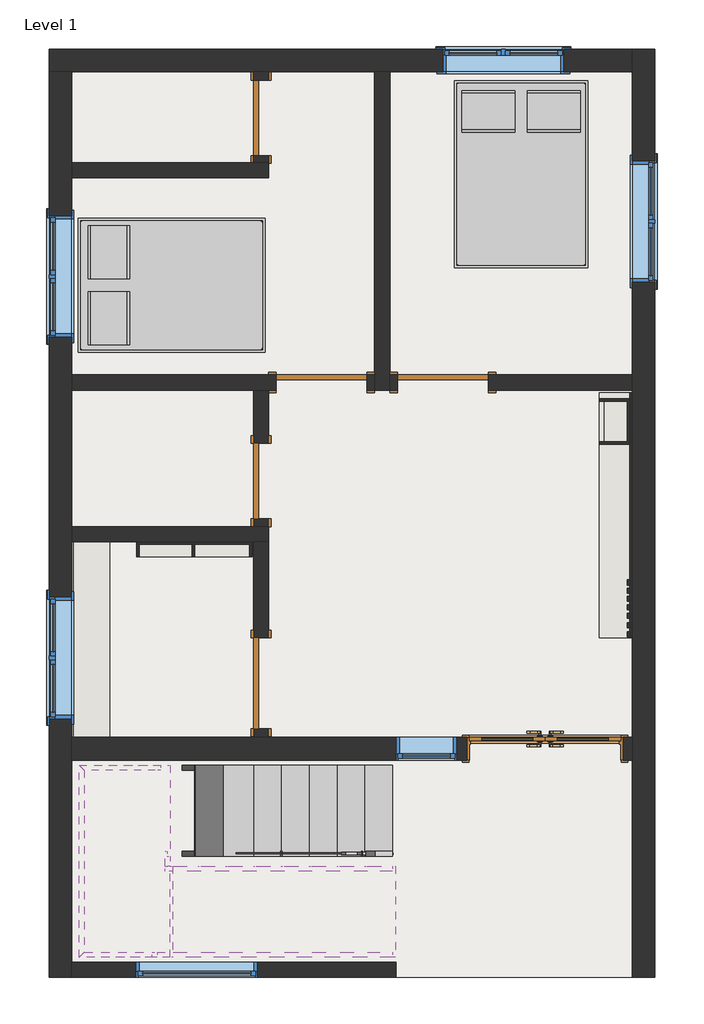
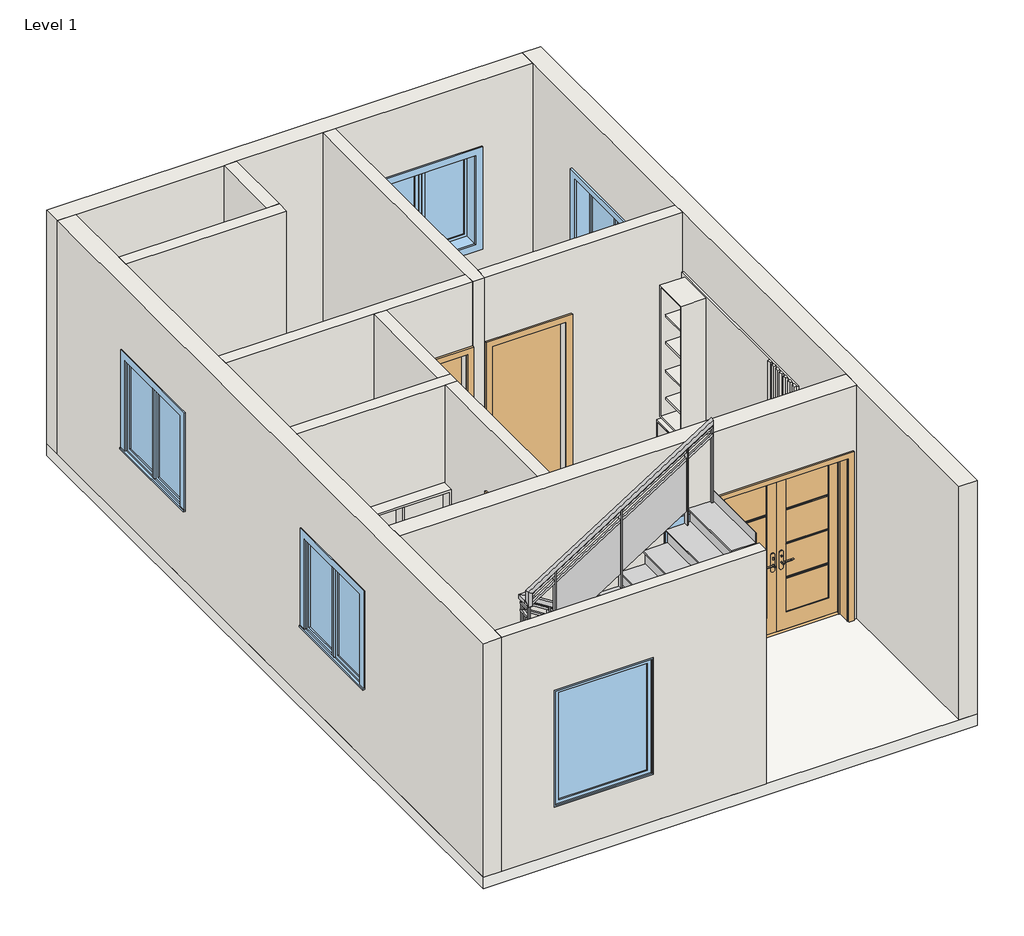
# One storey: 15 walls, 8 members, 6 doors, 6 windows, 2 furniture elements, 2 slabs, 2 stair flights, 1 railing.
"""IFC4 building model written with IfcOpenShell, lengths in millimetres."""

from ifc_helpers import new_model, si_unit, frame, origin, place, context, project, spatial, polyline, outline, extrude, faceted_brep, transform, mapped, element, save
from components import m_door_exterior_double_full_glass_wood_clad_1524_x_2134mm_606f56d5, single_flush_2_5_e2b13fe9, door_686f89d2, door_16372e1c, furniture_c8abb964, non_monolithic_landing_c2e345a4, stair_flight_0914375a, stair_flight_934fe551, walls_1_walls_1_7121089b, walls_2_walls_2_a3e54821, window_534dcd48, window_fc882ab3, fixed_4_86eadd64

model = new_model("IFC4")

# Units and contexts
model_context = context("Model", 3, world=origin())
ifc_project = project(units=[si_unit("LENGTHUNIT", "METRE", prefix="MILLI")], contexts=[model_context])

# Site, building, storey
site = spatial("IfcSite", under=ifc_project)
building = spatial("IfcBuilding", under=site)
storey = spatial("IfcBuildingStorey", under=building, Name="Level 1", Elevation=0.0)

# Doors
placement = place(None, origin())
m_door_exterior_double_full_glass_wood_clad_1524_x_2134mm_shape = m_door_exterior_double_full_glass_wood_clad_1524_x_2134mm_606f56d5(model_context)
element("IfcDoor", 1, ObjectType="M_Door-Exterior-Double-Full Glass-Wood_Clad : 1524 x 2134mm", at=placement, inside=storey, context=model_context, shape_type="MappedRepresentation", body=[
    mapped(m_door_exterior_double_full_glass_wood_clad_1524_x_2134mm_shape, transform((-1710.6681702, -4701.782676, 0.0), x_axis=(1.0, 0.0, 0.0), y_axis=(0.0, 1.0, 0.0), z_axis=(0.0, 0.0, 1.0))),
])
single_flush_2_5_shape = single_flush_2_5_e2b13fe9(model_context)
element("IfcDoor", 2, ObjectType="Single-Flush : 2.5'", at=placement, inside=storey, context=model_context, shape_type="MappedRepresentation", body=[
    mapped(single_flush_2_5_shape, transform((-4568.1681702, -2012.557676, 0.0), x_axis=(0.0, -1.0, 0.0), y_axis=(1.0, 0.0, 0.0), z_axis=(0.0, 0.0, 1.0))),
])
element("IfcDoor", 3, ObjectType="Single-Flush : 2.5'", at=placement, inside=storey, context=model_context, shape_type="MappedRepresentation", body=[
    mapped(single_flush_2_5_shape, transform((-4568.1681702, 1638.692324, 0.0), x_axis=(0.0, -1.0, 0.0), y_axis=(1.0, 0.0, 0.0), z_axis=(0.0, 0.0, 1.0))),
])
door_shape = door_686f89d2(model_context)
element("IfcDoor", 4, ObjectType="Single-Flush : 36\" x 84\"", at=placement, inside=storey, context=model_context, shape_type="MappedRepresentation", body=[
    mapped(door_shape, transform((-4568.1681702, -4044.557676, 0.0), x_axis=(0.0, -1.0, 0.0), y_axis=(1.0, 0.0, 0.0), z_axis=(0.0, 0.0, 1.0))),
])
element("IfcDoor", 5, ObjectType="Single-Flush : 36\" x 84\"", at=placement, inside=storey, context=model_context, shape_type="MappedRepresentation", body=[
    mapped(door_shape, transform((-2739.3681702, -1021.957676, 0.0), x_axis=(-1.0, 0.0, 0.0), y_axis=(0.0, -1.0, 0.0), z_axis=(0.0, 0.0, 1.0))),
])
door_2_shape = door_16372e1c(model_context)
element("IfcDoor", 6, ObjectType="Single-Flush : 36\" x 84\"", at=placement, inside=storey, context=model_context, shape_type="MappedRepresentation", body=[
    mapped(door_2_shape, transform((-3958.5681702, -1021.957676, 0.0), x_axis=(1.0, 0.0, 0.0), y_axis=(0.0, 1.0, 0.0), z_axis=(0.0, 0.0, 1.0))),
])

# Furniture
furniture_shape = furniture_c8abb964(model_context)
element("IfcFurniture", 7, ObjectType="Bed-Box : Double 53\" x 74\"", at=placement, inside=storey, context=model_context, shape_type="MappedRepresentation", body=[
    mapped(furniture_shape, transform((-5704.2976784, -383.210135, 0.0), x_axis=(0.0, 0.9999999999999999, 0.0), y_axis=(-0.9999999999999999, 0.0, 0.0), z_axis=(0.0, 0.0, 1.0))),
])
element("IfcFurniture", 8, ObjectType="Bed-Box : Double 53\" x 74\"", at=placement, inside=storey, context=model_context, shape_type="MappedRepresentation", body=[
    mapped(furniture_shape, transform((-2291.1206292, 1307.9718322, 0.0), x_axis=(1.0, 0.0, 0.0), y_axis=(0.0, 1.0, 0.0), z_axis=(0.0, 0.0, 1.0))),
])

# Members
element("IfcMember", 9, ObjectType="Carriage - 2\" Width", at=placement, inside=storey, context=model_context, shape_type="Brep", body=[
    faceted_brep([(-3247.3681702, -5936.857676, 2876.3282995), (-3247.3681702, -5886.057676, 2876.3282995), (-3247.3681702, -5886.057676, 2971.8), (-3247.3681702, -5936.857676, 2971.8), (-3495.0181702, -5886.057676, 2718.732845), (-3774.4181702, -5886.057676, 2540.932845), (-4053.8181702, -5886.057676, 2363.132845), (-4333.2181702, -5886.057676, 2185.332845), (-4612.6181702, -5886.057676, 2007.532845), (-4892.0181702, -5886.057676, 1829.732845), (-5171.4181702, -5886.057676, 1651.932845), (-5450.8181702, -5886.057676, 1474.132845), (-5482.5681702, -5886.057676, 1453.9282995), (-5533.3681702, -5886.057676, 1421.6010268), (-5533.3681702, -5886.057676, 1549.4), (-5482.5681702, -5886.057676, 1549.4), (-5450.8181702, -5886.057676, 1549.4), (-5450.8181702, -5886.057676, 1727.2), (-5171.4181702, -5886.057676, 1727.2), (-5171.4181702, -5886.057676, 1905.0), (-4892.0181702, -5886.057676, 1905.0), (-4892.0181702, -5886.057676, 2082.8), (-4612.6181702, -5886.057676, 2082.8), (-4612.6181702, -5886.057676, 2260.6), (-4333.2181702, -5886.057676, 2260.6), (-4333.2181702, -5886.057676, 2438.4), (-4053.8181702, -5886.057676, 2438.4), (-4053.8181702, -5886.057676, 2616.2), (-3774.4181702, -5886.057676, 2616.2), (-3774.4181702, -5886.057676, 2794.0), (-3495.0181702, -5886.057676, 2794.0), (-3495.0181702, -5886.057676, 2971.8), (-5533.3681702, -5936.857676, 1421.6010268), (-3495.0181702, -5936.857676, 2971.8), (-3495.0181702, -5936.857676, 2794.0), (-3774.4181702, -5936.857676, 2794.0), (-3774.4181702, -5936.857676, 2616.2), (-4053.8181702, -5936.857676, 2616.2), (-4053.8181702, -5936.857676, 2438.4), (-4333.2181702, -5936.857676, 2438.4), (-4333.2181702, -5936.857676, 2260.6), (-4612.6181702, -5936.857676, 2260.6), (-4612.6181702, -5936.857676, 2082.8), (-4892.0181702, -5936.857676, 2082.8), (-4892.0181702, -5936.857676, 1905.0), (-5171.4181702, -5936.857676, 1905.0), (-5171.4181702, -5936.857676, 1727.2), (-5450.8181702, -5936.857676, 1727.2), (-5450.8181702, -5936.857676, 1549.4), (-5533.3681702, -5936.857676, 1549.4)], [[[0, 1, 2, 3]], [[2, 1, 4, 5, 6, 7, 8, 9, 10, 11, 12, 13, 14, 15, 16, 17, 18, 19, 20, 21, 22, 23, 24, 25, 26, 27, 28, 29, 30, 31]], [[1, 0, 32, 13, 12, 11, 10, 9, 8, 7, 6, 5, 4]], [[32, 0, 3, 33, 34, 35, 36, 37, 38, 39, 40, 41, 42, 43, 44, 45, 46, 47, 48, 49]], [[17, 47, 46, 18]], [[47, 17, 16, 48]], [[19, 45, 44, 20]], [[18, 46, 45, 19]], [[21, 43, 42, 22]], [[20, 44, 43, 21]], [[23, 41, 40, 24]], [[22, 42, 41, 23]], [[25, 39, 38, 26]], [[24, 40, 39, 25]], [[27, 37, 36, 28]], [[26, 38, 37, 27]], [[29, 35, 34, 30]], [[28, 36, 35, 29]], [[31, 33, 3, 2]], [[30, 34, 33, 31]], [[13, 32, 49, 14]], [[48, 16, 15, 14, 49]]]),
])
element("IfcMember", 10, ObjectType="Carriage - 2\" Width", at=placement, inside=storey, context=model_context, shape_type="Brep", body=[
    faceted_brep([(-3247.3681702, -6800.457676, 2876.3282995), (-3247.3681702, -6749.657676, 2876.3282995), (-3247.3681702, -6749.657676, 2971.8), (-3247.3681702, -6800.457676, 2971.8), (-5611.9412123, -6749.657676, 1371.6), (-5663.7166945, -6749.657676, 1549.4), (-5450.8181702, -6749.657676, 1549.4), (-5450.8181702, -6749.657676, 1727.2), (-5171.4181702, -6749.657676, 1727.2), (-5171.4181702, -6749.657676, 1905.0), (-4892.0181702, -6749.657676, 1905.0), (-4892.0181702, -6749.657676, 2082.8), (-4612.6181702, -6749.657676, 2082.8), (-4612.6181702, -6749.657676, 2260.6), (-4333.2181702, -6749.657676, 2260.6), (-4333.2181702, -6749.657676, 2438.4), (-4053.8181702, -6749.657676, 2438.4), (-4053.8181702, -6749.657676, 2616.2), (-3774.4181702, -6749.657676, 2616.2), (-3774.4181702, -6749.657676, 2794.0), (-3495.0181702, -6749.657676, 2794.0), (-3495.0181702, -6749.657676, 2971.8), (-3495.0181702, -6800.457676, 2718.732845), (-3774.4181702, -6800.457676, 2540.932845), (-4053.8181702, -6800.457676, 2363.132845), (-4333.2181702, -6800.457676, 2185.332845), (-4612.6181702, -6800.457676, 2007.532845), (-4892.0181702, -6800.457676, 1829.732845), (-5171.4181702, -6800.457676, 1651.932845), (-5450.8181702, -6800.457676, 1474.132845), (-5482.5681702, -6800.457676, 1453.9282995), (-5611.9412123, -6800.457676, 1371.6), (-3495.0181702, -6800.457676, 2971.8), (-3495.0181702, -6800.457676, 2794.0), (-3774.4181702, -6800.457676, 2794.0), (-3774.4181702, -6800.457676, 2616.2), (-4053.8181702, -6800.457676, 2616.2), (-4053.8181702, -6800.457676, 2438.4), (-4333.2181702, -6800.457676, 2438.4), (-4333.2181702, -6800.457676, 2260.6), (-4612.6181702, -6800.457676, 2260.6), (-4612.6181702, -6800.457676, 2082.8), (-4892.0181702, -6800.457676, 2082.8), (-4892.0181702, -6800.457676, 1905.0), (-5171.4181702, -6800.457676, 1905.0), (-5171.4181702, -6800.457676, 1727.2), (-5450.8181702, -6800.457676, 1727.2), (-5450.8181702, -6800.457676, 1549.4), (-5482.5681702, -6800.457676, 1549.4), (-5663.7166945, -6800.457676, 1549.4)], [[[0, 1, 2, 3]], [[1, 4, 5, 6, 7, 8, 9, 10, 11, 12, 13, 14, 15, 16, 17, 18, 19, 20, 21, 2]], [[1, 0, 22, 23, 24, 25, 26, 27, 28, 29, 30, 31, 4]], [[0, 3, 32, 33, 34, 35, 36, 37, 38, 39, 40, 41, 42, 43, 44, 45, 46, 47, 48, 49, 31, 30, 29, 28, 27, 26, 25, 24, 23, 22]], [[7, 46, 45, 8]], [[46, 7, 6, 47]], [[9, 44, 43, 10]], [[8, 45, 44, 9]], [[11, 42, 41, 12]], [[10, 43, 42, 11]], [[13, 40, 39, 14]], [[12, 41, 40, 13]], [[15, 38, 37, 16]], [[14, 39, 38, 15]], [[17, 36, 35, 18]], [[16, 37, 36, 17]], [[19, 34, 33, 20]], [[18, 35, 34, 19]], [[21, 32, 3, 2]], [[20, 33, 32, 21]], [[4, 31, 49, 5]], [[47, 6, 5, 49, 48]]]),
])
element("IfcMember", 11, ObjectType="Carriage - 2\" Width", at=placement, inside=storey, context=model_context, shape_type="Brep", body=[
    faceted_brep([(-3279.1181702, -5784.457676, 0.0), (-3477.2236996, -5784.457676, 0.0), (-3477.2236996, -5733.657676, 0.0), (-3279.1181702, -5733.657676, 0.0), (-5482.5681702, -5784.457676, 1276.1282995), (-5482.5681702, -5733.657676, 1276.1282995), (-3558.5181702, -5784.457676, 51.732845), (-3837.9181702, -5784.457676, 229.532845), (-4117.3181702, -5784.457676, 407.332845), (-4396.7181702, -5784.457676, 585.132845), (-4676.1181702, -5784.457676, 762.932845), (-4955.5181702, -5784.457676, 940.732845), (-5234.9181702, -5784.457676, 1118.532845), (-5482.5681702, -5784.457676, 1371.6), (-3279.1181702, -5784.457676, 127.0), (-3558.5181702, -5784.457676, 127.0), (-3558.5181702, -5784.457676, 304.8), (-3837.9181702, -5784.457676, 304.8), (-3837.9181702, -5784.457676, 482.6), (-4117.3181702, -5784.457676, 482.6), (-4117.3181702, -5784.457676, 660.4), (-4396.7181702, -5784.457676, 660.4), (-4396.7181702, -5784.457676, 838.2), (-4676.1181702, -5784.457676, 838.2), (-4676.1181702, -5784.457676, 1016.0), (-4955.5181702, -5784.457676, 1016.0), (-4955.5181702, -5784.457676, 1193.8), (-5234.9181702, -5784.457676, 1193.8), (-5234.9181702, -5784.457676, 1371.6), (-5234.9181702, -5733.657676, 1371.6), (-5482.5681702, -5733.657676, 1371.6), (-5234.9181702, -5733.657676, 1193.8), (-4955.5181702, -5733.657676, 1193.8), (-4955.5181702, -5733.657676, 1016.0), (-4676.1181702, -5733.657676, 1016.0), (-4676.1181702, -5733.657676, 838.2), (-4396.7181702, -5733.657676, 838.2), (-4396.7181702, -5733.657676, 660.4), (-4117.3181702, -5733.657676, 660.4), (-4117.3181702, -5733.657676, 482.6), (-3837.9181702, -5733.657676, 482.6), (-3837.9181702, -5733.657676, 304.8), (-3558.5181702, -5733.657676, 304.8), (-3558.5181702, -5733.657676, 127.0), (-3279.1181702, -5733.657676, 127.0)], [[[0, 1, 2, 3]], [[4, 5, 2, 1, 6, 7, 8, 9, 10, 11, 12]], [[13, 4, 12, 11, 10, 9, 8, 7, 6, 1, 0, 14, 15, 16, 17, 18, 19, 20, 21, 22, 23, 24, 25, 26, 27, 28]], [[28, 29, 30, 13]], [[2, 5, 30, 29, 31, 32, 33, 34, 35, 36, 37, 38, 39, 40, 41, 42, 43, 44, 3]], [[44, 14, 0, 3]], [[14, 44, 43, 15]], [[15, 43, 42, 16]], [[16, 42, 41, 17]], [[17, 41, 40, 18]], [[18, 40, 39, 19]], [[19, 39, 38, 20]], [[20, 38, 37, 21]], [[21, 37, 36, 22]], [[22, 36, 35, 23]], [[23, 35, 34, 24]], [[24, 34, 33, 25]], [[25, 33, 32, 26]], [[26, 32, 31, 27]], [[27, 31, 29, 28]], [[5, 4, 13, 30]]]),
])
element("IfcMember", 12, ObjectType="Carriage - 2\" Width", at=placement, inside=storey, context=model_context, shape_type="Brep", body=[
    faceted_brep([(-3279.1181702, -4920.857676, 0.0), (-3477.2236996, -4920.857676, 0.0), (-3477.2236996, -4870.057676, 0.0), (-3279.1181702, -4870.057676, 0.0), (-5632.5951281, -4920.857676, 1371.6), (-5632.5951281, -4870.057676, 1371.6), (-5514.3181702, -4870.057676, 1296.332845), (-5482.5681702, -4870.057676, 1276.1282995), (-5234.9181702, -4870.057676, 1118.532845), (-4955.5181702, -4870.057676, 940.732845), (-4676.1181702, -4870.057676, 762.932845), (-4396.7181702, -4870.057676, 585.132845), (-4117.3181702, -4870.057676, 407.332845), (-3837.9181702, -4870.057676, 229.532845), (-3558.5181702, -4870.057676, 51.732845), (-5580.8196459, -4920.857676, 1549.4), (-3279.1181702, -4920.857676, 127.0), (-3558.5181702, -4920.857676, 127.0), (-3558.5181702, -4920.857676, 304.8), (-3837.9181702, -4920.857676, 304.8), (-3837.9181702, -4920.857676, 482.6), (-4117.3181702, -4920.857676, 482.6), (-4117.3181702, -4920.857676, 660.4), (-4396.7181702, -4920.857676, 660.4), (-4396.7181702, -4920.857676, 838.2), (-4676.1181702, -4920.857676, 838.2), (-4676.1181702, -4920.857676, 1016.0), (-4955.5181702, -4920.857676, 1016.0), (-4955.5181702, -4920.857676, 1193.8), (-5234.9181702, -4920.857676, 1193.8), (-5234.9181702, -4920.857676, 1371.6), (-5514.3181702, -4920.857676, 1371.6), (-5514.3181702, -4920.857676, 1549.4), (-5234.9181702, -4870.057676, 1371.6), (-5482.5681702, -4870.057676, 1371.6), (-5514.3181702, -4870.057676, 1371.6), (-5580.8196459, -4870.057676, 1549.4), (-5514.3181702, -4870.057676, 1549.4), (-5234.9181702, -4870.057676, 1193.8), (-4955.5181702, -4870.057676, 1193.8), (-4955.5181702, -4870.057676, 1016.0), (-4676.1181702, -4870.057676, 1016.0), (-4676.1181702, -4870.057676, 838.2), (-4396.7181702, -4870.057676, 838.2), (-4396.7181702, -4870.057676, 660.4), (-4117.3181702, -4870.057676, 660.4), (-4117.3181702, -4870.057676, 482.6), (-3837.9181702, -4870.057676, 482.6), (-3837.9181702, -4870.057676, 304.8), (-3558.5181702, -4870.057676, 304.8), (-3558.5181702, -4870.057676, 127.0), (-3279.1181702, -4870.057676, 127.0)], [[[0, 1, 2, 3]], [[4, 5, 6, 7, 8, 9, 10, 11, 12, 13, 14, 2, 1]], [[15, 4, 1, 0, 16, 17, 18, 19, 20, 21, 22, 23, 24, 25, 26, 27, 28, 29, 30, 31, 32]], [[30, 33, 34, 35, 31]], [[5, 36, 37, 35, 34, 33, 38, 39, 40, 41, 42, 43, 44, 45, 46, 47, 48, 49, 50, 51, 3, 2, 14, 13, 12, 11, 10, 9, 8, 7, 6]], [[51, 16, 0, 3]], [[16, 51, 50, 17]], [[17, 50, 49, 18]], [[18, 49, 48, 19]], [[19, 48, 47, 20]], [[20, 47, 46, 21]], [[21, 46, 45, 22]], [[22, 45, 44, 23]], [[23, 44, 43, 24]], [[24, 43, 42, 25]], [[25, 42, 41, 26]], [[26, 41, 40, 27]], [[27, 40, 39, 28]], [[28, 39, 38, 29]], [[29, 38, 33, 30]], [[5, 4, 15, 36]], [[31, 35, 37, 32]], [[32, 37, 36, 15]]]),
])
element("IfcMember", 13, ObjectType="Carriage - 2\" Width", at=placement, inside=storey, context=model_context, shape_type="SweptSolid", body=[
    extrude(outline(polyline([(-5533.3681702, -5886.057676), (-5533.3681702, -5733.657676), (-5514.3181702, -5733.657676), (-5514.3181702, -5784.457676), (-5482.5681702, -5784.457676), (-5482.5681702, -5886.057676), (-5533.3681702, -5886.057676)])), frame((0.0, 0.0, 1371.6), z_axis=(0.0, 0.0, 1.0), x_axis=(1.0, 0.0, 0.0)), (0.0, 0.0, 1.0), 177.8),
])
element("IfcMember", 14, ObjectType="Carriage - 2\" Width", at=placement, inside=storey, context=model_context, shape_type="Brep", body=[
    faceted_brep([(-6346.1681702, -4920.857676, 1371.6), (-5632.5951281, -4920.857676, 1371.6), (-5580.8196459, -4920.857676, 1549.4), (-6346.1681702, -4920.857676, 1549.4), (-6396.9681702, -4870.057676, 1371.6), (-5632.5951281, -4870.057676, 1371.6), (-6396.9681702, -4870.057676, 1549.4), (-5580.8196459, -4870.057676, 1549.4)], [[[0, 1, 2, 3]], [[1, 0, 4, 5]], [[5, 4, 6, 7]], [[3, 2, 7, 6]], [[1, 5, 7, 2]], [[4, 0, 3, 6]]]),
])
element("IfcMember", 15, ObjectType="Carriage - 2\" Width", at=placement, inside=storey, context=model_context, shape_type="SweptSolid", body=[
    extrude(outline(polyline([(-6346.1681702, -4920.857676), (-6346.1681702, -6749.657676), (-6396.9681702, -6800.457676), (-6396.9681702, -4870.057676), (-6346.1681702, -4920.857676)])), frame((0.0, 0.0, 1371.6), z_axis=(0.0, 0.0, 1.0), x_axis=(1.0, 0.0, 0.0)), (0.0, 0.0, 1.0), 177.8),
])
element("IfcMember", 16, ObjectType="Carriage - 2\" Width", at=placement, inside=storey, context=model_context, shape_type="Brep", body=[
    faceted_brep([(-5611.9412123, -6749.657676, 1371.6), (-6346.1681702, -6749.657676, 1371.6), (-6346.1681702, -6749.657676, 1549.4), (-5663.7166945, -6749.657676, 1549.4), (-5611.9412123, -6800.457676, 1371.6), (-6396.9681702, -6800.457676, 1371.6), (-5663.7166945, -6800.457676, 1549.4), (-6396.9681702, -6800.457676, 1549.4)], [[[0, 1, 2, 3]], [[1, 0, 4, 5]], [[5, 4, 6, 7]], [[3, 2, 7, 6]], [[1, 5, 7, 2]], [[4, 0, 3, 6]]]),
])

# Railing
element("IfcRailing", 17, ObjectType="Glass Panel - Bottom Fill", at=placement, inside=storey, context=model_context, shape_type="SolidModel", body=[
    faceted_brep([(-5533.3681702, -5886.057676, 2660.0727273), (-5482.5681702, -5886.057676, 2632.186276), (-5482.5681702, -5936.857676, 2632.186276), (-5533.3681702, -5936.857676, 2660.0727273), (-3247.3681702, -5886.057676, 4114.8), (-3247.3681702, -5936.857676, 4114.8), (-3247.3681702, -5936.857676, 4054.586276), (-3247.3681702, -5886.057676, 4054.586276)], [[[0, 1, 2, 3]], [[4, 5, 6, 7]], [[1, 0, 4, 7]], [[2, 1, 7, 6]], [[3, 2, 6, 5]], [[0, 3, 5, 4]]]),
    faceted_brep([(-5482.5681702, -5886.057676, 2514.6), (-5533.3681702, -5886.057676, 2514.6), (-5533.3681702, -5936.857676, 2463.8), (-5482.5681702, -5936.857676, 2463.8), (-5482.5681702, -5860.657676, 2463.8), (-5482.5681702, -5860.657676, 2514.6), (-5533.3681702, -5860.657676, 2463.8), (-5533.3681702, -5860.657676, 2514.6), (-3247.3681702, -5784.457676, 1092.2), (-3247.3681702, -5784.457676, 1031.986276), (-3247.3681702, -5733.657676, 1031.986276), (-3247.3681702, -5733.657676, 1092.2), (-5406.3681702, -5784.457676, 2466.1090909), (-5457.1681702, -5784.457676, 2438.2226396), (-5457.1681702, -5733.657676, 2438.2226396), (-5406.3681702, -5733.657676, 2466.1090909), (-5406.3681702, -5784.457676, 2514.6), (-5457.1681702, -5784.457676, 2463.8), (-5457.1681702, -5733.657676, 2463.8), (-5406.3681702, -5733.657676, 2514.6), (-5482.5681702, -5784.457676, 2514.6), (-5482.5681702, -5784.457676, 2463.8), (-5533.3681702, -5733.657676, 2463.8), (-5533.3681702, -5733.657676, 2514.6)], [[[0, 1, 2, 3]], [[4, 5, 0, 3]], [[6, 4, 3, 2]], [[7, 6, 2, 1]], [[5, 7, 1, 0]], [[8, 9, 10, 11]], [[9, 8, 12, 13]], [[10, 9, 13, 14]], [[11, 10, 14, 15]], [[8, 11, 15, 12]], [[13, 12, 16, 17]], [[14, 13, 17, 18]], [[15, 14, 18, 19]], [[12, 15, 19, 16]], [[17, 16, 20, 21]], [[18, 17, 21, 22]], [[19, 18, 22, 23]], [[16, 19, 23, 20]], [[21, 20, 5, 4]], [[22, 21, 4, 6]], [[23, 22, 6, 7]], [[20, 23, 7, 5]]]),
    faceted_brep([(-5482.5681702, -5886.057676, 2514.6), (-5482.5681702, -5936.857676, 2463.8), (-5533.3681702, -5936.857676, 2463.8), (-5533.3681702, -5886.057676, 2514.6), (-5482.5681702, -5886.057676, 2632.186276), (-5533.3681702, -5886.057676, 2660.0727273), (-5533.3681702, -5936.857676, 2660.0727273), (-5482.5681702, -5936.857676, 2632.186276)], [[[0, 1, 2, 3]], [[4, 5, 6, 7]], [[1, 0, 4, 7]], [[2, 1, 7, 6]], [[3, 2, 6, 5]], [[0, 3, 5, 4]]]),
    faceted_brep([(-3247.3681702, -5771.757676, 1005.653431), (-3247.3681702, -5771.757676, 975.546569), (-3247.3681702, -5746.357676, 975.546569), (-3247.3681702, -5746.357676, 1005.653431), (-5478.8699215, -5771.757676, 2425.7), (-5486.2664189, -5771.757676, 2400.3), (-5486.2664189, -5746.357676, 2400.3), (-5478.8699215, -5746.357676, 2425.7), (-5495.2681702, -5771.757676, 2425.7), (-5495.2681702, -5771.757676, 2400.3), (-5520.6681702, -5746.357676, 2400.3), (-5520.6681702, -5746.357676, 2425.7), (-5495.2681702, -5898.757676, 2425.7), (-5520.6681702, -5898.757676, 2425.7), (-5520.6681702, -5898.757676, 2400.3), (-5495.2681702, -5898.757676, 2400.3)], [[[0, 1, 2, 3]], [[1, 0, 4, 5]], [[2, 1, 5, 6]], [[3, 2, 6, 7]], [[0, 3, 7, 4]], [[5, 4, 8, 9]], [[6, 5, 9, 10]], [[7, 6, 10, 11]], [[4, 7, 11, 8]], [[12, 13, 14, 15]], [[9, 8, 12, 15]], [[10, 9, 15, 14]], [[11, 10, 14, 13]], [[8, 11, 13, 12]]]),
    faceted_brep([(-5520.6681702, -5898.757676, 2581.6079765), (-5520.6681702, -5898.757676, 2551.5011144), (-5520.6681702, -5924.157676, 2551.5011144), (-5520.6681702, -5924.157676, 2581.6079765), (-3247.3681702, -5898.757676, 4028.253431), (-3247.3681702, -5924.157676, 4028.253431), (-3247.3681702, -5924.157676, 3998.146569), (-3247.3681702, -5898.757676, 3998.146569)], [[[0, 1, 2, 3]], [[4, 5, 6, 7]], [[1, 0, 4, 7]], [[2, 1, 7, 6]], [[3, 2, 6, 5]], [[0, 3, 5, 4]]]),
    faceted_brep([(-3247.3681702, -5771.757676, 904.053431), (-3247.3681702, -5771.757676, 873.946569), (-3247.3681702, -5746.357676, 873.946569), (-3247.3681702, -5746.357676, 904.053431), (-5478.8699215, -5771.757676, 2324.1), (-5486.2664189, -5771.757676, 2298.7), (-5486.2664189, -5746.357676, 2298.7), (-5478.8699215, -5746.357676, 2324.1), (-5495.2681702, -5771.757676, 2324.1), (-5495.2681702, -5771.757676, 2298.7), (-5520.6681702, -5746.357676, 2298.7), (-5520.6681702, -5746.357676, 2324.1), (-5495.2681702, -5898.757676, 2324.1), (-5520.6681702, -5898.757676, 2324.1), (-5520.6681702, -5898.757676, 2298.7), (-5495.2681702, -5898.757676, 2298.7)], [[[0, 1, 2, 3]], [[1, 0, 4, 5]], [[2, 1, 5, 6]], [[3, 2, 6, 7]], [[0, 3, 7, 4]], [[5, 4, 8, 9]], [[6, 5, 9, 10]], [[7, 6, 10, 11]], [[4, 7, 11, 8]], [[12, 13, 14, 15]], [[9, 8, 12, 15]], [[10, 9, 15, 14]], [[11, 10, 14, 13]], [[8, 11, 13, 12]]]),
    faceted_brep([(-5520.6681702, -5898.757676, 2480.0079765), (-5520.6681702, -5898.757676, 2449.9011144), (-5520.6681702, -5924.157676, 2449.9011144), (-5520.6681702, -5924.157676, 2480.0079765), (-3247.3681702, -5898.757676, 3926.653431), (-3247.3681702, -5924.157676, 3926.653431), (-3247.3681702, -5924.157676, 3896.546569), (-3247.3681702, -5898.757676, 3896.546569)], [[[0, 1, 2, 3]], [[4, 5, 6, 7]], [[1, 0, 4, 7]], [[2, 1, 7, 6]], [[3, 2, 6, 5]], [[0, 3, 5, 4]]]),
    extrude(outline(polyline([(3848.4999123, -3571.2181702), (2844.8, -3571.2181702), (2844.8, -3558.5181702), (3856.5817305, -3558.5181702), (3848.4999123, -3571.2181702)])), frame((0.0, -5936.857676, 0.0), z_axis=(0.0, 1.0, 0.0), x_axis=(0.0, 0.0, 1.0)), (0.0, 0.0, 1.0), 50.8),
    extrude(outline(polyline([(2509.9818182, -4377.6681702), (3027.2181818, -3564.8681702), (3694.5011144, -3564.8681702), (3177.2647508, -4377.6681702), (2509.9818182, -4377.6681702)])), frame((0.0, -5917.992833, 0.0), z_axis=(0.0, 1.0, 0.0), x_axis=(0.0, 0.0, 1.0)), (0.0, 0.0, 1.0), 6.35),
    extrude(outline(polyline([(3331.2635487, -4384.0181702), (2311.4, -4384.0181702), (2311.4, -4371.3181702), (3339.3453669, -4371.3181702), (3331.2635487, -4384.0181702)])), frame((0.0, -5936.857676, 0.0), z_axis=(0.0, 1.0, 0.0), x_axis=(0.0, 0.0, 1.0)), (0.0, 0.0, 1.0), 50.8),
    extrude(outline(polyline([(1976.5818182, -5190.4681702), (2493.8181818, -4377.6681702), (3177.2647508, -4377.6681702), (2660.0283872, -5190.4681702), (1976.5818182, -5190.4681702)])), frame((0.0, -5917.992833, 0.0), z_axis=(0.0, 1.0, 0.0), x_axis=(0.0, 0.0, 1.0)), (0.0, 0.0, 1.0), 6.35),
    extrude(outline(polyline([(2814.0271851, -5196.8181702), (1955.8, -5196.8181702), (1955.8, -5184.1181702), (2822.1090032, -5184.1181702), (2814.0271851, -5196.8181702)])), frame((0.0, -5936.857676, 0.0), z_axis=(0.0, 1.0, 0.0), x_axis=(0.0, 0.0, 1.0)), (0.0, 0.0, 1.0), 50.8),
    extrude(outline(polyline([(2264.4635487, -5184.1181702), (1244.6, -5184.1181702), (1244.6, -5171.4181702), (2256.3817305, -5171.4181702), (2264.4635487, -5184.1181702)])), frame((0.0, -5784.457676, 0.0), z_axis=(0.0, 1.0, 0.0), x_axis=(0.0, 0.0, 1.0)), (0.0, 0.0, 1.0), 50.8),
    extrude(outline(polyline([(909.7818182, -4364.9681702), (1585.146569, -4364.9681702), (2102.3829326, -5177.7681702), (1427.0181818, -5177.7681702), (909.7818182, -4364.9681702)])), frame((0.0, -5758.872519, 0.0), z_axis=(0.0, 1.0, 0.0), x_axis=(0.0, 0.0, 1.0)), (0.0, 0.0, 1.0), 6.35),
    extrude(outline(polyline([(1747.2271851, -4371.3181702), (889.0, -4371.3181702), (889.0, -4358.6181702), (1739.1453669, -4358.6181702), (1747.2271851, -4371.3181702)])), frame((0.0, -5784.457676, 0.0), z_axis=(0.0, 1.0, 0.0), x_axis=(0.0, 0.0, 1.0)), (0.0, 0.0, 1.0), 50.8),
    extrude(outline(polyline([(376.3818182, -3552.1681702), (1067.9102054, -3552.1681702), (1585.146569, -4364.9681702), (893.6181818, -4364.9681702), (376.3818182, -3552.1681702)])), frame((0.0, -5758.872519, 0.0), z_axis=(0.0, 1.0, 0.0), x_axis=(0.0, 0.0, 1.0)), (0.0, 0.0, 1.0), 6.35),
    extrude(outline(polyline([(1229.9908214, -3558.5181702), (355.6, -3558.5181702), (355.6, -3545.8181702), (1221.9090032, -3545.8181702), (1229.9908214, -3558.5181702)])), frame((0.0, -5784.457676, 0.0), z_axis=(0.0, 1.0, 0.0), x_axis=(0.0, 0.0, 1.0)), (0.0, 0.0, 1.0), 50.8),
    extrude(outline(polyline([(-5517.4931702, -5901.932676), (-5498.4431702, -5901.932676), (-5498.4431702, -5920.982676), (-5517.4931702, -5920.982676), (-5517.4931702, -5901.932676)])), frame((0.0, 0.0, 1600.2), z_axis=(0.0, 0.0, 1.0), x_axis=(1.0, 0.0, 0.0)), (0.0, 0.0, 1.0), 863.6),
    extrude(outline(polyline([(-5498.4431702, -5768.582676), (-5517.4931702, -5768.582676), (-5517.4931702, -5749.532676), (-5498.4431702, -5749.532676), (-5498.4431702, -5768.582676)])), frame((0.0, 0.0, 1600.2), z_axis=(0.0, 0.0, 1.0), x_axis=(1.0, 0.0, 0.0)), (0.0, 0.0, 1.0), 863.6),
    extrude(outline(polyline([(-5473.0431702, -5768.582676), (-5492.0931702, -5768.582676), (-5492.0931702, -5749.532676), (-5473.0431702, -5749.532676), (-5473.0431702, -5768.582676)])), frame((0.0, 0.0, 1600.2), z_axis=(0.0, 0.0, 1.0), x_axis=(1.0, 0.0, 0.0)), (0.0, 0.0, 1.0), 863.6),
    extrude(outline(polyline([(4046.5044578, -3260.0681702), (3022.6, -3260.0681702), (3022.6, -3241.0181702), (4058.6271851, -3241.0181702), (4046.5044578, -3260.0681702)])), frame((0.0, -5920.982676, 0.0), z_axis=(0.0, 1.0, 0.0), x_axis=(0.0, 0.0, 1.0)), (0.0, 0.0, 1.0), 19.05),
    extrude(outline(polyline([(1040.0680941, -3260.0681702), (177.8, -3260.0681702), (177.8, -3241.0181702), (1027.9453669, -3241.0181702), (1040.0680941, -3260.0681702)])), frame((0.0, -5768.582676, 0.0), z_axis=(0.0, 1.0, 0.0), x_axis=(0.0, 0.0, 1.0)), (0.0, 0.0, 1.0), 19.05),
])

# Slabs
element("IfcSlab", 18, ObjectType="6\"", at=placement, inside=storey, context=model_context, shape_type="SweptSolid", body=[
    extrude(outline(polyline([(-605.7681702, 2330.842324), (-605.7681702, -7003.657676), (-6701.7681702, -7003.657676), (-6701.7681702, 2330.842324), (-605.7681702, 2330.842324)])), frame((0.0, 0.0, -152.4), z_axis=(0.0, 0.0, 1.0), x_axis=(1.0, 0.0, 0.0)), (0.0, 0.0, 1.0), 152.4),
])
non_monolithic_landing_shape = non_monolithic_landing_c2e345a4(model_context)
element("IfcSlab", 19, ObjectType="Non-Monolithic Landing", at=placement, inside=storey, context=model_context, shape_type="MappedRepresentation", body=[
    mapped(non_monolithic_landing_shape, transform((0.0, 0.0, 0.0), x_axis=(1.0, 0.0, 0.0), y_axis=(0.0, 1.0, 0.0), z_axis=(0.0, 0.0, 1.0))),
])

# Stair flights
stair_flight_shape = stair_flight_0914375a(model_context)
element("IfcStairFlight", 20, ObjectType="2\" Tread 1\" Nosing 1/4\" Riser", at=placement, inside=storey, context=model_context, shape_type="MappedRepresentation", body=[
    mapped(stair_flight_shape, transform((0.0, 0.0, 0.0), x_axis=(1.0, 0.0, 0.0), y_axis=(0.0, 1.0, 0.0), z_axis=(0.0, 0.0, 1.0))),
])
stair_flight_2_shape = stair_flight_934fe551(model_context)
element("IfcStairFlight", 21, ObjectType="2\" Tread 1\" Nosing 1/4\" Riser", at=placement, inside=storey, context=model_context, shape_type="MappedRepresentation", body=[
    mapped(stair_flight_2_shape, transform((0.0, 0.0, 0.0), x_axis=(1.0, 0.0, 0.0), y_axis=(0.0, 1.0, 0.0), z_axis=(0.0, 0.0, 1.0))),
])

# Walls
element("IfcWall", 22, ObjectType="6\"", at=placement, inside=storey, context=model_context, shape_type="Brep", body=[
    faceted_brep([(-3425.1681702, 2102.242324, 0.0), (-3425.1681702, -945.757676, 0.0), (-3425.1681702, -1098.157676, 0.0), (-3425.1681702, -1098.157676, 3048.0), (-3425.1681702, -945.757676, 3048.0), (-3425.1681702, 2102.242324, 3048.0), (-3272.7681702, 2102.242324, 0.0), (-3272.7681702, 2102.242324, 3048.0), (-3272.7681702, -945.757676, 3048.0), (-3272.7681702, -1098.157676, 3048.0), (-3272.7681702, -1098.157676, 0.0), (-3272.7681702, -945.757676, 0.0)], [[[0, 1, 2, 3, 4, 5]], [[6, 7, 8, 9, 10, 11]], [[2, 1, 0, 6, 11, 10]], [[5, 4, 3, 9, 8, 7]], [[0, 5, 7, 6]], [[3, 2, 10, 9]]]),
])
element("IfcWall", 23, ObjectType="6\"", at=placement, inside=storey, context=model_context, shape_type="Brep", body=[
    faceted_brep([(-3425.1681702, -945.757676, 0.0), (-3501.3681702, -945.757676, 0.0), (-3501.3681702, -945.757676, 2133.6), (-4415.7681702, -945.757676, 2133.6), (-4415.7681702, -945.757676, 0.0), (-6473.1681702, -945.757676, 0.0), (-6473.1681702, -945.757676, 3048.0), (-3425.1681702, -945.757676, 3048.0), (-3501.3681702, -1098.157676, 2133.6), (-3501.3681702, -1098.157676, 0.0), (-3425.1681702, -1098.157676, 0.0), (-3425.1681702, -1098.157676, 3048.0), (-4491.9681702, -1098.157676, 3048.0), (-4644.3681702, -1098.157676, 3048.0), (-6473.1681702, -1098.157676, 3048.0), (-6473.1681702, -1098.157676, 0.0), (-4644.3681702, -1098.157676, 0.0), (-4491.9681702, -1098.157676, 0.0), (-4415.7681702, -1098.157676, 0.0), (-4415.7681702, -1098.157676, 2133.6)], [[[0, 1, 2, 3, 4, 5, 6, 7]], [[8, 9, 10, 11, 12, 13, 14, 15, 16, 17, 18, 19]], [[10, 9, 1, 0]], [[18, 17, 16, 15, 5, 4]], [[7, 6, 14, 13, 12, 11]], [[6, 5, 15, 14]], [[0, 7, 11, 10]], [[2, 1, 9, 8]], [[3, 2, 8, 19]], [[4, 3, 19, 18]]]),
])
element("IfcWall", 24, ObjectType="6\"", at=placement, inside=storey, context=model_context, shape_type="SweptSolid", body=[
    extrude(outline(polyline([(0.0, -3272.7681702), (0.0, -3196.5681702), (2133.6, -3196.5681702), (2133.6, -2282.1681702), (0.0, -2282.1681702), (0.0, -834.3681702), (3048.0, -834.3681702), (3048.0, -3272.7681702), (0.0, -3272.7681702)])), frame((0.0, -1098.157676, 0.0), z_axis=(0.0, 1.0, 0.0), x_axis=(0.0, 0.0, 1.0)), (0.0, 0.0, 1.0), 152.4),
])
element("IfcWall", 25, ObjectType="6\"", at=placement, inside=storey, context=model_context, shape_type="Brep", body=[
    faceted_brep([(-6473.1681702, -2622.157676, 0.0), (-4644.3681702, -2622.157676, 0.0), (-4491.9681702, -2622.157676, 0.0), (-4491.9681702, -2622.157676, 3048.0), (-4644.3681702, -2622.157676, 3048.0), (-6473.1681702, -2622.157676, 3048.0), (-6473.1681702, -2469.757676, 0.0), (-6473.1681702, -2469.757676, 3048.0), (-4644.3681702, -2469.757676, 3048.0), (-4491.9681702, -2469.757676, 3048.0), (-4491.9681702, -2469.757676, 0.0), (-4644.3681702, -2469.757676, 0.0)], [[[0, 1, 2, 3, 4, 5]], [[6, 7, 8, 9, 10, 11]], [[2, 1, 0, 6, 11, 10]], [[5, 4, 3, 9, 8, 7]], [[0, 5, 7, 6]], [[3, 2, 10, 9]]]),
])
element("IfcWall", 26, ObjectType="6\"", at=placement, inside=storey, context=model_context, shape_type="SweptSolid", body=[
    extrude(outline(polyline([(-2393.557676, 2133.6), (-2393.557676, 0.0), (-2469.757676, 0.0), (-2469.757676, 3048.0), (-1098.157676, 3048.0), (-1098.157676, 0.0), (-1631.557676, 0.0), (-1631.557676, 2133.6), (-2393.557676, 2133.6)])), frame((-4644.3681702, 0.0, 0.0), z_axis=(1.0, 0.0, 0.0), x_axis=(0.0, 1.0, 0.0)), (0.0, 0.0, 1.0), 152.4),
])
element("IfcWall", 27, ObjectType="6\"", at=placement, inside=storey, context=model_context, shape_type="SweptSolid", body=[
    extrude(outline(polyline([(-4501.757676, 2133.6), (-4501.757676, 0.0), (-4590.657676, 0.0), (-4590.657676, 3048.0), (-2622.157676, 3048.0), (-2622.157676, 0.0), (-3587.357676, 0.0), (-3587.357676, 2133.6), (-4501.757676, 2133.6)])), frame((-4644.3681702, 0.0, 0.0), z_axis=(1.0, 0.0, 0.0), x_axis=(0.0, 1.0, 0.0)), (0.0, 0.0, 1.0), 152.4),
])
element("IfcWall", 28, ObjectType="6\"", at=placement, inside=storey, context=model_context, shape_type="SweptSolid", body=[
    extrude(outline(polyline([(1257.692324, 2133.6), (1257.692324, 0.0), (1187.842324, 0.0), (1187.842324, 3048.0), (2102.242324, 3048.0), (2102.242324, 0.0), (2019.692324, 0.0), (2019.692324, 2133.6), (1257.692324, 2133.6)])), frame((-4644.3681702, 0.0, 0.0), z_axis=(1.0, 0.0, 0.0), x_axis=(0.0, 1.0, 0.0)), (0.0, 0.0, 1.0), 152.4),
])
element("IfcWall", 29, ObjectType="6\"", at=placement, inside=storey, context=model_context, shape_type="Brep", body=[
    faceted_brep([(-4491.9681702, 1187.842324, 0.0), (-4644.3681702, 1187.842324, 0.0), (-6473.1681702, 1187.842324, 0.0), (-6473.1681702, 1187.842324, 3048.0), (-4644.3681702, 1187.842324, 3048.0), (-4491.9681702, 1187.842324, 3048.0), (-4491.9681702, 1035.442324, 0.0), (-4491.9681702, 1035.442324, 3048.0), (-6473.1681702, 1035.442324, 3048.0), (-6473.1681702, 1035.442324, 0.0)], [[[0, 1, 2, 3, 4, 5]], [[6, 7, 8, 9]], [[2, 1, 0, 6, 9]], [[5, 4, 3, 8, 7]], [[3, 2, 9, 8]], [[0, 5, 7, 6]]]),
])
element("IfcWall", 30, ObjectType="6\"", at=placement, inside=storey, context=model_context, shape_type="SweptSolid", body=[
    extrude(outline(polyline([(0.0, -3209.2681702), (3048.0, -3209.2681702), (3048.0, -6473.1681702), (0.0, -6473.1681702), (0.0, -3209.2681702)]), holes=[polyline([(2133.6, -5825.4681702), (2133.6, -4606.2681702), (609.6, -4606.2681702), (609.6, -5825.4681702), (2133.6, -5825.4681702)])]), frame((0.0, -7003.657676, 0.0), z_axis=(0.0, 1.0, 0.0), x_axis=(0.0, 0.0, 1.0)), (0.0, 0.0, 1.0), 152.4),
])
element("IfcWall", 31, ObjectType="9\"", at=placement, inside=storey, context=model_context, shape_type="Brep", body=[
    faceted_brep([(-6701.7681702, 2102.242324, 0.0), (-6473.1681702, 2102.242324, 0.0), (-4644.3681702, 2102.242324, 0.0), (-4491.9681702, 2102.242324, 0.0), (-3425.1681702, 2102.242324, 0.0), (-3272.7681702, 2102.242324, 0.0), (-834.3681702, 2102.242324, 0.0), (-834.3681702, 2102.242324, 3048.0), (-3272.7681702, 2102.242324, 3048.0), (-3425.1681702, 2102.242324, 3048.0), (-4491.9681702, 2102.242324, 3048.0), (-4644.3681702, 2102.242324, 3048.0), (-6473.1681702, 2102.242324, 3048.0), (-6701.7681702, 2102.242324, 3048.0), (-1520.1681702, 2102.242324, 2133.6), (-1520.1681702, 2102.242324, 914.4), (-2739.3681702, 2102.242324, 914.4), (-2739.3681702, 2102.242324, 2133.6), (-6701.7681702, 2330.842324, 0.0), (-6701.7681702, 2330.842324, 3048.0), (-834.3681702, 2330.842324, 3048.0), (-834.3681702, 2330.842324, 0.0), (-1520.1681702, 2330.842324, 2133.6), (-2739.3681702, 2330.842324, 2133.6), (-2739.3681702, 2330.842324, 914.4), (-1520.1681702, 2330.842324, 914.4)], [[[0, 1, 2, 3, 4, 5, 6, 7, 8, 9, 10, 11, 12, 13], [14, 15, 16, 17]], [[18, 19, 20, 21], [22, 23, 24, 25]], [[6, 5, 4, 3, 2, 1, 0, 18, 21]], [[13, 12, 11, 10, 9, 8, 7, 20, 19]], [[0, 13, 19, 18]], [[7, 6, 21, 20]], [[15, 14, 22, 25]], [[16, 15, 25, 24]], [[17, 16, 24, 23]], [[14, 17, 23, 22]]]),
])
element("IfcWall", 32, ObjectType="9\"", at=placement, inside=storey, context=model_context, shape_type="Brep", body=[
    faceted_brep([(-6473.1681702, -7003.657676, 0.0), (-6473.1681702, -6851.257676, 0.0), (-6473.1681702, -4819.257676, 0.0), (-6473.1681702, -4590.657676, 0.0), (-6473.1681702, -2622.157676, 0.0), (-6473.1681702, -2469.757676, 0.0), (-6473.1681702, -1098.157676, 0.0), (-6473.1681702, -945.757676, 0.0), (-6473.1681702, 1035.442324, 0.0), (-6473.1681702, 1187.842324, 0.0), (-6473.1681702, 2102.242324, 0.0), (-6473.1681702, 2102.242324, 3048.0), (-6473.1681702, 1187.842324, 3048.0), (-6473.1681702, 1035.442324, 3048.0), (-6473.1681702, -945.757676, 3048.0), (-6473.1681702, -1098.157676, 3048.0), (-6473.1681702, -2469.757676, 3048.0), (-6473.1681702, -2622.157676, 3048.0), (-6473.1681702, -4590.657676, 3048.0), (-6473.1681702, -4819.257676, 3048.0), (-6473.1681702, -6851.257676, 3048.0), (-6473.1681702, -7003.657676, 3048.0), (-6473.1681702, -3180.957676, 2133.6), (-6473.1681702, -3180.957676, 914.4), (-6473.1681702, -4400.157676, 914.4), (-6473.1681702, -4400.157676, 2133.6), (-6473.1681702, 654.442324, 2133.6), (-6473.1681702, 654.442324, 914.4), (-6473.1681702, -564.757676, 914.4), (-6473.1681702, -564.757676, 2133.6), (-6701.7681702, -7003.657676, 0.0), (-6701.7681702, -7003.657676, 3048.0), (-6701.7681702, 2102.242324, 3048.0), (-6701.7681702, 2102.242324, 0.0), (-6701.7681702, -3180.957676, 2133.6), (-6701.7681702, -4400.157676, 2133.6), (-6701.7681702, -4400.157676, 914.4), (-6701.7681702, -3180.957676, 914.4), (-6701.7681702, 654.442324, 2133.6), (-6701.7681702, -564.757676, 2133.6), (-6701.7681702, -564.757676, 914.4), (-6701.7681702, 654.442324, 914.4)], [[[0, 1, 2, 3, 4, 5, 6, 7, 8, 9, 10, 11, 12, 13, 14, 15, 16, 17, 18, 19, 20, 21], [22, 23, 24, 25], [26, 27, 28, 29]], [[30, 31, 32, 33], [34, 35, 36, 37], [38, 39, 40, 41]], [[10, 9, 8, 7, 6, 5, 4, 3, 2, 1, 0, 30, 33]], [[21, 20, 19, 18, 17, 16, 15, 14, 13, 12, 11, 32, 31]], [[0, 21, 31, 30]], [[11, 10, 33, 32]], [[23, 22, 34, 37]], [[24, 23, 37, 36]], [[25, 24, 36, 35]], [[22, 25, 35, 34]], [[27, 26, 38, 41]], [[28, 27, 41, 40]], [[29, 28, 40, 39]], [[26, 29, 39, 38]]]),
])
element("IfcWall", 33, ObjectType="9\"", at=placement, inside=storey, context=model_context, shape_type="Brep", body=[
    faceted_brep([(-834.3681702, 2330.842324, 0.0), (-834.3681702, 2102.242324, 0.0), (-834.3681702, -945.757676, 0.0), (-834.3681702, -1098.157676, 0.0), (-834.3681702, -4590.657676, 0.0), (-834.3681702, -4819.257676, 0.0), (-834.3681702, -7003.657676, 0.0), (-834.3681702, -7003.657676, 3048.0), (-834.3681702, -4819.257676, 3048.0), (-834.3681702, -4590.657676, 3048.0), (-834.3681702, -1098.157676, 3048.0), (-834.3681702, -945.757676, 3048.0), (-834.3681702, 2102.242324, 3048.0), (-834.3681702, 2330.842324, 3048.0), (-834.3681702, -12.307676, 2133.6), (-834.3681702, -12.307676, 914.4), (-834.3681702, 1206.892324, 914.4), (-834.3681702, 1206.892324, 2133.6), (-605.7681702, 2330.842324, 0.0), (-605.7681702, 2330.842324, 3048.0), (-605.7681702, -7003.657676, 3048.0), (-605.7681702, -7003.657676, 0.0), (-605.7681702, -12.307676, 2133.6), (-605.7681702, 1206.892324, 2133.6), (-605.7681702, 1206.892324, 914.4), (-605.7681702, -12.307676, 914.4)], [[[0, 1, 2, 3, 4, 5, 6, 7, 8, 9, 10, 11, 12, 13], [14, 15, 16, 17]], [[18, 19, 20, 21], [22, 23, 24, 25]], [[6, 5, 4, 3, 2, 1, 0, 18, 21]], [[7, 6, 21, 20]], [[13, 12, 11, 10, 9, 8, 7, 20, 19]], [[0, 13, 19, 18]], [[15, 14, 22, 25]], [[16, 15, 25, 24]], [[17, 16, 24, 23]], [[14, 17, 23, 22]]]),
])
element("IfcWall", 34, ObjectType="9\"", at=placement, inside=storey, context=model_context, shape_type="Brep", body=[
    faceted_brep([(-834.3681702, -4819.257676, 3048.0), (-6473.1681702, -4819.257676, 3048.0), (-6473.1681702, -4819.257676, 0.0), (-2497.6681702, -4819.257676, 0.0), (-2497.6681702, -4819.257676, 2158.6), (-923.6681702, -4819.257676, 2158.6), (-923.6681702, -4819.257676, 0.0), (-834.3681702, -4819.257676, 0.0), (-3209.2681702, -4819.257676, 2133.6), (-2599.6681702, -4819.257676, 2133.6), (-2599.6681702, -4819.257676, 304.8), (-3209.2681702, -4819.257676, 304.8), (-6473.1681702, -4590.657676, 3048.0), (-4644.3681702, -4590.657676, 3048.0), (-4491.9681702, -4590.657676, 3048.0), (-834.3681702, -4590.657676, 3048.0), (-834.3681702, -4590.657676, 0.0), (-923.6681702, -4590.657676, 0.0), (-923.6681702, -4590.657676, 2158.6), (-2497.6681702, -4590.657676, 2158.6), (-2497.6681702, -4590.657676, 0.0), (-4491.9681702, -4590.657676, 0.0), (-4644.3681702, -4590.657676, 0.0), (-6473.1681702, -4590.657676, 0.0), (-3209.2681702, -4590.657676, 2133.6), (-3209.2681702, -4590.657676, 304.8), (-2599.6681702, -4590.657676, 304.8), (-2599.6681702, -4590.657676, 2133.6)], [[[0, 1, 2, 3, 4, 5, 6, 7], [8, 9, 10, 11]], [[12, 13, 14, 15, 16, 17, 18, 19, 20, 21, 22, 23], [24, 25, 26, 27]], [[2, 23, 22, 21, 20, 3]], [[16, 7, 6, 17]], [[1, 0, 15, 14, 13, 12]], [[2, 1, 12, 23]], [[0, 7, 16, 15]], [[5, 18, 17, 6]], [[18, 5, 4, 19]], [[19, 4, 3, 20]], [[25, 24, 8, 11]], [[26, 25, 11, 10]], [[27, 26, 10, 9]], [[24, 27, 9, 8]]]),
])
walls_1_walls_1_shape = walls_1_walls_1_7121089b(model_context)
element("IfcWall", 35, ObjectType="Walls 1 : Walls 1", at=placement, inside=storey, context=model_context, shape_type="MappedRepresentation", body=[
    mapped(walls_1_walls_1_shape, transform((0.0, 0.0, 0.0), x_axis=(1.0, 0.0, 0.0), y_axis=(0.0, 1.0, 0.0), z_axis=(0.0, 0.0, 1.0))),
])
walls_2_walls_2_shape = walls_2_walls_2_a3e54821(model_context)
element("IfcWall", 36, ObjectType="Walls 2 : Walls 2", at=placement, inside=storey, context=model_context, shape_type="MappedRepresentation", body=[
    mapped(walls_2_walls_2_shape, transform((0.0, 0.0, 0.0), x_axis=(1.0, 0.0, 0.0), y_axis=(0.0, 1.0, 0.0), z_axis=(0.0, 0.0, 1.0))),
])

# Windows
window_shape = window_534dcd48(model_context)
element("IfcWindow", 37, ObjectType="Casement Dbl with Trim : 48\" x 48\"", at=placement, inside=storey, context=model_context, shape_type="MappedRepresentation", body=[
    mapped(window_shape, transform((-6568.4181702, -3790.557676, 0.0), x_axis=(0.0, 1.0, 0.0), y_axis=(-1.0, 0.0, 0.0), z_axis=(0.0, 0.0, 1.0))),
])
element("IfcWindow", 38, ObjectType="Casement Dbl with Trim : 48\" x 48\"", at=placement, inside=storey, context=model_context, shape_type="MappedRepresentation", body=[
    mapped(window_shape, transform((-739.1181702, 597.292324, 0.0), x_axis=(0.0, -1.0, 0.0), y_axis=(1.0, 0.0, 0.0), z_axis=(0.0, 0.0, 1.0))),
])
element("IfcWindow", 39, ObjectType="Casement Dbl with Trim : 48\" x 48\"", at=placement, inside=storey, context=model_context, shape_type="MappedRepresentation", body=[
    mapped(window_shape, transform((-2129.7681702, 2197.492324, 0.0), x_axis=(1.0, 0.0, 0.0), y_axis=(0.0, 1.0, 0.0), z_axis=(0.0, 0.0, 1.0))),
])
element("IfcWindow", 40, ObjectType="Casement Dbl with Trim : 48\" x 48\"", at=placement, inside=storey, context=model_context, shape_type="MappedRepresentation", body=[
    mapped(window_shape, transform((-6568.4181702, 44.842324, 0.0), x_axis=(0.0, 1.0, 0.0), y_axis=(-1.0, 0.0, 0.0), z_axis=(0.0, 0.0, 1.0))),
])
window_2_shape = window_fc882ab3(model_context)
element("IfcWindow", 41, ObjectType="Fixed : 24\" x 72\"", at=placement, inside=storey, context=model_context, shape_type="MappedRepresentation", body=[
    mapped(window_2_shape, transform((-2942.5681702, -4704.957676, 0.0), x_axis=(-1.0, 0.0, 0.0), y_axis=(0.0, -1.0, 0.0), z_axis=(0.0, 0.0, 1.0))),
])
fixed_4_shape = fixed_4_86eadd64(model_context)
element("IfcWindow", 42, ObjectType="Fixed : 4'", at=placement, inside=storey, context=model_context, shape_type="MappedRepresentation", body=[
    mapped(fixed_4_shape, transform((-5253.9681702, -6927.457676, 0.0), x_axis=(-1.0, 0.0, 0.0), y_axis=(0.0, -1.0, 0.0), z_axis=(0.0, 0.0, 1.0))),
])

save(model, "model.ifc")

# Revit data of these elements
# Type "M_Door-Exterior-Double-Full Glass-Wood_Clad : 1524 x 2134mm"
#   Type Mark = "9"
#   Assembly Code = "B2030100"
#   Analytic Construction = "French door, wood frame with double glass"
#   Top Rail = 0' - 4.72441"
#   Threshold Offset [instance default] = 0' - 0.59055"
#   Thickness = 0' - 1.37795"
#   Thermal Resistance (R) = 1.9158 (h·ft²·°F)/BTU
#   Swing Angle [instance default] = 90.00°
#   Stiles = 0' - 4.72441"
#   Rough Width = 5' - 1.9685"
#   Rough Height = 7' - 0.98425"
#   Panel Width = 2' - 6"
#   Door Offset [instance default] = 0' - 0"
#   Height = 7' - 0"
#   Width = 5' - 0"
#   Heat Transfer Coefficient (U) = 0.5220 BTU/(h·ft²·°F)
#   Bottom Rail = 0' - 9.05512"
#   Exterior Trim [instance default] = yes
#   Threshold [instance default] = yes
#   Show Grill [instance default] = yes
#   Function = 1
#   Trim Material = Cherry
#   Threshold Material = Cherry
#   Panel Material = Cherry
#   Glazing = Glass
#   Frame Material = Cherry
#   Door Handle Material = Aluminum
#   Visual Light Transmittance = 0
#   Solar Heat Gain Coefficient = 0
#   Wall Closure = (empty or 0)
#   Construction Type = (empty or 0)
# Type "Single-Flush : 2.5'"
#   Type Mark = "8"
#   Construction Type Id = "MDOOR"
#   Assembly Code = "C1020"
#   Analytic Construction = "Metal"
#   Thickness = 0' - 2"
#   Heat Transfer Coefficient (U) = 0.651978 BTU/(h·ft²·°F)
#   Height = 7' - 0"
#   Trim Projection Ext = 0' - 1"
#   Trim Projection Int = 0' - 1"
#   Trim Width = 0' - 3"
#   Width = 2' - 6"
#   Define Thermal Properties by = 1
#   Door Material = Door - Panel
#   Frame Material = Door - Frame
#   Visual Light Transmittance = 0
#   Solar Heat Gain Coefficient = 0
#   Function = (empty or 0)
#   Wall Closure = (empty or 0)
# Type "Single-Flush : 36\" x 84\""
#   Type Mark = "1"
#   Construction Type Id = "MDOOR"
#   Assembly Code = "C1020"
#   Analytic Construction = "Metal"
#   Thickness = 0' - 2"
#   Heat Transfer Coefficient (U) = 0.651978 BTU/(h·ft²·°F)
#   Height = 7' - 0"
#   Trim Projection Ext = 0' - 1"
#   Trim Projection Int = 0' - 1"
#   Trim Width = 0' - 3"
#   Width = 3' - 0"
#   Define Thermal Properties by = 1
#   Door Material = Door - Panel
#   Frame Material = Door - Frame
#   Visual Light Transmittance = 0
#   Solar Heat Gain Coefficient = 0
#   Function = (empty or 0)
#   Wall Closure = (empty or 0)
# Type "Bed-Box : Double 53\" x 74\""
#   Assembly Code = "E2020200"
#   Length = 6' - 2"
#   Width = 4' - 5"
#   Frame Material = Birch
#   Mattress Material = Linen, White
#   Default Elevation = 0
# Type "Glass Panel - Bottom Fill"
#   Assembly Code = "C2010400"
#   built-in parameter 1008612 = 0.0416667 (stored number, unit not read)
#   built-in parameter 1008611 = 0.0416667 (stored number, unit not read)
#   built-in parameter 1008609 = 0.333333 (stored number, unit not read)
#   built-in parameter 1008604 = 0.166667 (stored number, unit not read)
#   built-in parameter 1008603 = 0.166667 (stored number, unit not read)
#   Railing Height = 3' - 0"
#   built-in parameter 1008630 = 2
#   built-in parameter 1008610 = 2
#   built-in parameter 1008618 = Baluster - Square : 3/4"
# Type "6\""
#   Assembly Code = "B1010"
#   Function = 0
#   Layers, outside or top first: 0' - 6" "floor" (function 1)
# Type "6\""
#   Assembly Code = "B2010"
#   Layers, outside or top first: 0' - 6" "ext wall" (function 1)
# Type "9\""
#   Assembly Code = "B2010"
#   Layers, outside or top first: 0' - 9" "int wall" (function 1)
# Type "Casement Dbl with Trim : 48\" x 48\""
#   Type Mark = "10"
#   Construction Type Id = "GSP4R"
#   Assembly Code = "B2020100"
#   Analytic Construction = "1/8 in Pilkington single glazing"
#   Visual Light Transmittance = 0.9
#   Solar Heat Gain Coefficient = 0.78
#   Heat Transfer Coefficient (U) = 0.6496 BTU/(h·ft²·°F)
#   Height = 4' - 0"
#   Default Sill Height = 3' - 0"
#   Trim Projection - Ext. = 0' - 0 1/2"
#   Trim Projection - Int. = 0' - 0 3/4"
#   Trim Width - Exterior = 0' - 3 1/2"
#   Trim Width - Interior = 0' - 3 1/2"
#   Width = 4' - 0"
#   Window Inset = 0' - 0 3/4"
#   Define Thermal Properties by = 1
#   Glass Pane Material = Glass
#   Sash Material = Sash
#   Trim Exterior Material = Trim
#   Trim Interior Material = Trim
#   Wall Closure = (empty or 0)
# Type "Fixed : 24\" x 72\""
#   Type Mark = "7"
#   Construction Type Id = "GSP4R"
#   Assembly Code = "B2020100"
#   Analytic Construction = "1/8 in Pilkington single glazing"
#   Visual Light Transmittance = 0.9
#   Solar Heat Gain Coefficient = 0.78
#   Heat Transfer Coefficient (U) = 0.6496 BTU/(h·ft²·°F)
#   Height = 6' - 0"
#   Default Sill Height = 1' - 0"
#   Width = 2' - 0"
#   Window Inset = 0' - 0 3/4"
#   Define Thermal Properties by = 1
#   Glass Pane Material = Glass
#   Sash Material = Sash
#   Wall Closure = (empty or 0)
# Type "Fixed : 4'"
#   Type Mark = "13"
#   Construction Type Id = "GSP4R"
#   Assembly Code = "B2020100"
#   Analytic Construction = "1/8 in Pilkington single glazing"
#   Visual Light Transmittance = 0.9
#   Solar Heat Gain Coefficient = 0.78
#   Heat Transfer Coefficient (U) = 0.6496 BTU/(h·ft²·°F)
#   Height = 5' - 0"
#   Default Sill Height = 2' - 0"
#   Width = 4' - 0"
#   Window Inset = 0' - 0 3/4"
#   Define Thermal Properties by = 1
#   Glass Pane Material = Glass
#   Sash Material = Sash
#   Wall Closure = (empty or 0)
# Element 1 (IfcDoor, "M_Door-Exterior-Double-Full Glass-Wood_Clad : 1524 x 2134mm")
#   Threshold Offset = 0' - 0.59055"
#   Swing Angle = 90.00°
#   Door Offset = 0' - 0"
#   Threshold = yes
#   Show Grill = yes
#   Exterior Trim = yes
#   Phase Created = New Construction
#   Materials on its faces: "Cherry", "Aluminum", "Glass"
# Elements 2, 3 (IfcDoor, "Single-Flush : 2.5'")
#   Phase Created = New Construction
#   Materials on its faces: "Door - Frame", "Door - Panel"
# Elements 4, 5, 6 (IfcDoor, "Single-Flush : 36\" x 84\"")
#   Phase Created = New Construction
#   Materials on its faces: "Door - Frame", "Door - Panel"
# Elements 7, 8 (IfcFurniture, "Bed-Box : Double 53\" x 74\"")
#   Phase Created = New Construction
#   Materials on its faces: "Birch", "Linen, White"
# Elements 9, 10, 11, 12, 13, 14, 15, 16 (IfcMember, "Carriage - 2\" Width")
#   Phase Created = New Construction
# Element 17 (IfcRailing, "Glass Panel - Bottom Fill")
#   Phase Created = New Construction
#   Materials on its faces: "Glass"
# Element 18 (IfcSlab, "6\"")
#   Height Offset From Level = 0' - 0"
#   Phase Created = New Construction
#   Materials on its faces: "floor"
# Element 19 (IfcSlab, "Non-Monolithic Landing")
#   Phase Created = New Construction
# Elements 20, 21 (IfcStairFlight, "2\" Tread 1\" Nosing 1/4\" Riser")
#   Phase Created = New Construction
# Elements 22, 23, 24, 25, 26, 27, 28, 29, 30 (IfcWall, "6\"")
#   Top Offset = 0' - 0"
#   Base Offset = 0' - 0"
#   Unconnected Height = 10' - 0"
#   wall height = 10' - 0"
#   Phase Created = New Construction
#   Base Constraint = Level 1
#   Materials on its faces: "ext wall"
# Elements 31, 33, 34 (IfcWall, "9\"")
#   Top Offset = 0' - 0"
#   Base Offset = 0' - 0"
#   Unconnected Height = 10' - 0"
#   wall height = 10' - 0"
#   Phase Created = New Construction
#   Base Constraint = Level 1
#   Materials on its faces: "int wall"
# Element 32 (IfcWall, "9\"")
#   Top Offset = 0' - 0"
#   Base Offset = 0' - 0"
#   Unconnected Height = 10' - 0"
#   wall height = 10' - 0"
#   Phase Created = New Construction
#   Base Constraint = Level 1
#   Materials on its faces: "int wall", "ext wall"
# Element 35 (IfcWall, "Walls 1 : Walls 1")
#   Phase Created = New Construction
#   Materials on its faces: "drawers", "wood", "clear glass", "stone", "Default Wall"
# Element 36 (IfcWall, "Walls 2 : Walls 2")
#   Phase Created = New Construction
#   Materials on its faces: "drawers", "metal", "wood"
# Element 37 (IfcWindow, "Casement Dbl with Trim : 48\" x 48\"")
#   Mark = "1"
#   Phase Created = New Construction
#   Materials on its faces: "Sash", "Trim", "Glass"
# Element 38 (IfcWindow, "Casement Dbl with Trim : 48\" x 48\"")
#   Mark = "4"
#   Phase Created = New Construction
#   Materials on its faces: "Sash", "Trim", "Glass"
# Element 39 (IfcWindow, "Casement Dbl with Trim : 48\" x 48\"")
#   Mark = "5"
#   Phase Created = New Construction
#   Materials on its faces: "Sash", "Trim", "Glass"
# Element 40 (IfcWindow, "Casement Dbl with Trim : 48\" x 48\"")
#   Mark = "20"
#   Phase Created = New Construction
#   Materials on its faces: "Sash", "Trim", "Glass"
# Element 41 (IfcWindow, "Fixed : 24\" x 72\"")
#   Mark = "6"
